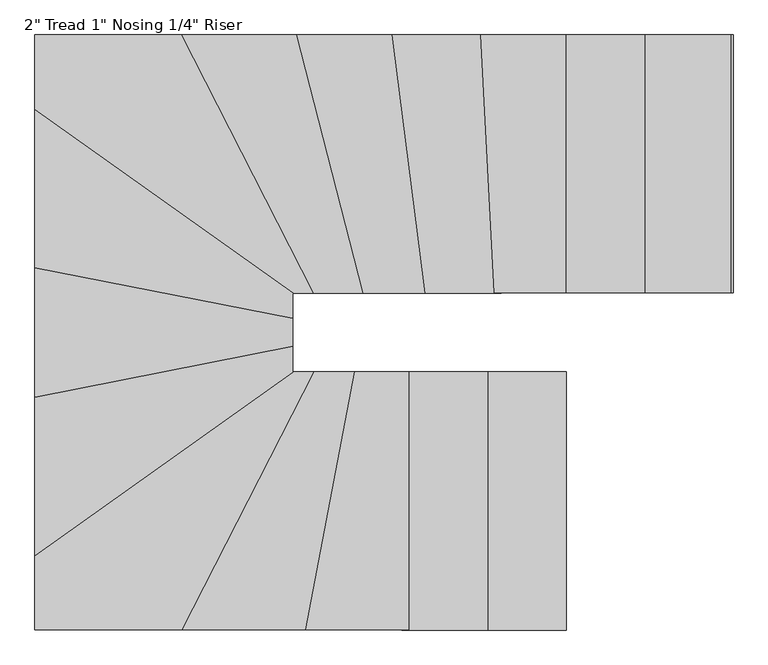
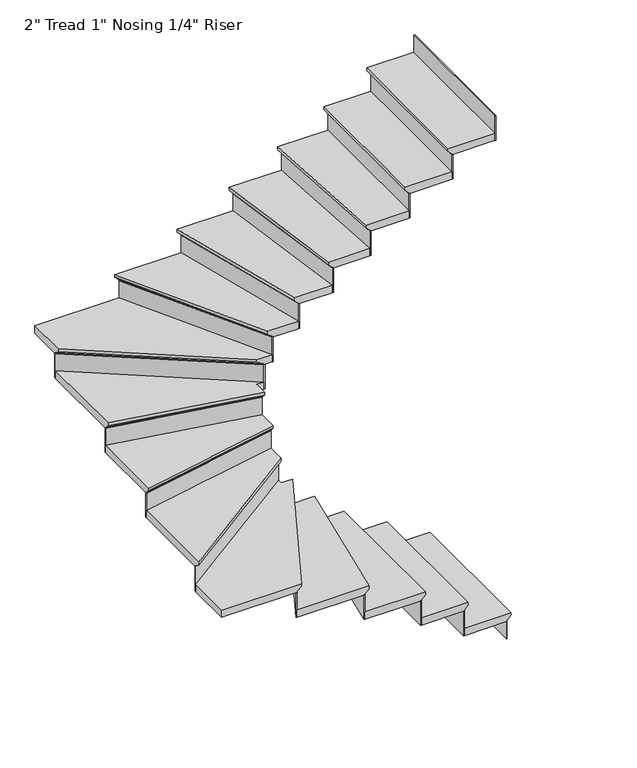
"""IFC4 building model written with IfcOpenShell, lengths in millimetres: stair flight geometry."""

from ifc_helpers import new_model, si_unit, origin, place, context, project, spatial, faceted_brep, source, transform, mapped, element, save


def stair_flight_5a50a9e8(model_context):
    return source(origin(), model_context, "Body", "Brep", [
        faceted_brep([(-8420.1659688, 2083.499435, 488.95), (-8420.1659688, 2083.499435, 508.0), (-8420.1659688, 1169.099435, 508.0), (-8420.1659688, 1169.099435, 488.95), (-8445.5659688, 2083.499435, 463.55), (-8445.5659688, 1169.099435, 463.55), (-8724.9659688, 2083.499435, 508.0), (-8724.9659688, 1169.099435, 508.0), (-8445.5659688, 1169.099435, 457.2), (-8724.9659688, 1169.099435, 457.2), (-8724.9659688, 2083.499435, 457.2), (-8445.5659688, 2083.499435, 457.2)], [[[0, 1, 2, 3]], [[4, 0, 3, 5]], [[2, 1, 6, 7]], [[8, 9, 10, 11]], [[2, 7, 9, 8, 5, 3]], [[8, 11, 4, 5]], [[6, 1, 0, 4, 11, 10]], [[7, 6, 10, 9]]]),
        faceted_brep([(-8445.5659688, 2083.499435, 457.2), (-8445.5659688, 2083.499435, 338.6666667), (-8451.9159688, 2083.499435, 338.6666667), (-8451.9159688, 2083.499435, 457.2), (-8445.5659688, 1169.099435, 457.2), (-8451.9159688, 1169.099435, 457.2), (-8451.9159688, 1169.099435, 338.6666667), (-8445.5659688, 1169.099435, 338.6666667)], [[[0, 1, 2, 3]], [[4, 5, 6, 7]], [[1, 0, 4, 7]], [[2, 1, 7, 6]], [[3, 2, 6, 5]], [[0, 3, 5, 4]]]),
        faceted_brep([(-8724.9659688, 2083.499435, 626.5333333), (-8724.9659688, 2083.499435, 457.2), (-8731.3159688, 2083.499435, 457.2), (-8731.3159688, 2083.499435, 626.5333333), (-8724.9659688, 1169.099435, 626.5333333), (-8731.3159688, 1169.099435, 626.5333333), (-8731.3159688, 1169.099435, 457.2), (-8724.9659688, 1169.099435, 457.2)], [[[0, 1, 2, 3]], [[4, 5, 6, 7]], [[1, 0, 4, 7]], [[2, 1, 7, 6]], [[3, 2, 6, 5]], [[0, 3, 5, 4]]]),
        faceted_brep([(-8699.5659688, 1169.099435, 677.3333333), (-8699.5659688, 2083.499435, 677.3333333), (-9004.3659688, 2083.499435, 677.3333333), (-9004.3659688, 1169.099435, 677.3333333), (-8724.9659688, 1169.099435, 626.5333333), (-9004.3659688, 1169.099435, 626.5333333), (-9004.3659688, 2083.499435, 626.5333333), (-8724.9659688, 2083.499435, 626.5333333), (-8724.9659688, 1169.099435, 632.8833333), (-8699.5659688, 1169.099435, 658.2833333), (-8724.9659688, 2083.499435, 632.8833333), (-8699.5659688, 2083.499435, 658.2833333)], [[[0, 1, 2, 3]], [[4, 5, 6, 7]], [[0, 3, 5, 4, 8, 9]], [[4, 7, 10, 8]], [[2, 1, 11, 10, 7, 6]], [[3, 2, 6, 5]], [[11, 1, 0, 9]], [[10, 11, 9, 8]]]),
        faceted_brep([(-9004.3659688, 2083.499435, 795.8666667), (-9004.3659688, 2083.499435, 626.5333333), (-9010.7159688, 2083.499435, 626.5333333), (-9010.7159688, 2083.499435, 795.8666667), (-9004.3659688, 1169.099435, 795.8666667), (-9010.7159688, 1169.099435, 795.8666667), (-9010.7159688, 1169.099435, 626.5333333), (-9004.3659688, 1169.099435, 626.5333333)], [[[0, 1, 2, 3]], [[4, 5, 6, 7]], [[1, 0, 4, 7]], [[2, 1, 7, 6]], [[3, 2, 6, 5]], [[0, 3, 5, 4]]]),
        faceted_brep([(-8978.9659688, 1169.099435, 846.6666667), (-8978.9659688, 2083.499435, 846.6666667), (-9197.7461084, 2083.499435, 846.6666667), (-9370.6864067, 1169.099435, 846.6666667), (-9004.3659688, 1169.099435, 795.8666667), (-9370.6864067, 1169.099435, 795.8666667), (-9197.7461084, 2083.499435, 795.8666667), (-9004.3659688, 2083.499435, 795.8666667), (-9004.3659688, 1169.099435, 802.2166667), (-8978.9659688, 1169.099435, 827.6166667), (-9004.3659688, 2083.499435, 802.2166667), (-8978.9659688, 2083.499435, 827.6166667)], [[[0, 1, 2, 3]], [[4, 5, 6, 7]], [[0, 3, 5, 4, 8, 9]], [[4, 7, 10, 8]], [[2, 1, 11, 10, 7, 6]], [[3, 2, 6, 5]], [[11, 1, 0, 9]], [[10, 11, 9, 8]]]),
        faceted_brep([(-9197.7461084, 2083.499435, 965.2), (-9197.7461084, 2083.499435, 795.8666667), (-9204.2086806, 2083.499435, 795.8666667), (-9204.2086806, 2083.499435, 965.2), (-9370.6864067, 1169.099435, 965.2), (-9377.1489789, 1169.099435, 965.2), (-9377.1489789, 1169.099435, 795.8666667), (-9370.6864067, 1169.099435, 795.8666667)], [[[0, 1, 2, 3]], [[4, 5, 6, 7]], [[1, 0, 4, 7]], [[2, 1, 7, 6]], [[3, 2, 6, 5]], [[0, 3, 5, 4]]]),
        faceted_brep([(-9344.836118, 1169.099435, 1016.0), (-9171.8958196, 2083.499435, 1016.0), (-9343.3736886, 2083.499435, 1016.0), (-9812.19831, 1169.099435, 1016.0), (-9370.6864067, 1169.099435, 965.2), (-9812.19831, 1169.099435, 965.2), (-9343.3736886, 2083.499435, 965.2), (-9197.7461084, 2083.499435, 965.2), (-9370.6864067, 1169.099435, 971.55), (-9344.836118, 1169.099435, 996.95), (-9197.7461084, 2083.499435, 971.55), (-9171.8958196, 2083.499435, 996.95)], [[[0, 1, 2, 3]], [[4, 5, 6, 7]], [[0, 3, 5, 4, 8, 9]], [[4, 7, 10, 8]], [[2, 1, 11, 10, 7, 6]], [[3, 2, 6, 5]], [[11, 1, 0, 9]], [[10, 11, 9, 8]]]),
        faceted_brep([(-9343.3736886, 2083.499435, 1134.5333333), (-9343.3736886, 2083.499435, 965.2), (-9350.5096718, 2083.499435, 965.2), (-9350.5096718, 2083.499435, 1134.5333333), (-9812.19831, 1169.099435, 1134.5333333), (-9819.3342931, 1169.099435, 1134.5333333), (-9819.3342931, 1169.099435, 965.2), (-9812.19831, 1169.099435, 965.2)], [[[0, 1, 2, 3]], [[4, 5, 6, 7]], [[1, 0, 4, 7]], [[2, 1, 7, 6]], [[3, 2, 6, 5]], [[0, 3, 5, 4]]]),
        faceted_brep([(-10303.4976606, 1462.7805687, 1185.3333333), (-10303.4976606, 1169.099435, 1185.3333333), (-9783.6543774, 1169.099435, 1185.3333333), (-9314.8297561, 2083.499435, 1185.3333333), (-9389.0976606, 2083.499435, 1185.3333333), (-9389.0976606, 2113.0545178, 1185.3333333), (-10303.4976606, 1169.099435, 1134.5333333), (-10303.4976606, 1462.7805687, 1134.5333333), (-9389.0976606, 2113.0545178, 1134.5333333), (-9389.0976606, 2083.499435, 1134.5333333), (-9343.3736886, 2083.499435, 1134.5333333), (-9812.19831, 1169.099435, 1134.5333333), (-9343.3736886, 2083.499435, 1140.8833333), (-9812.19831, 1169.099435, 1140.8833333), (-9314.8297561, 2083.499435, 1166.2833333), (-9783.6543774, 1169.099435, 1166.2833333)], [[[0, 1, 2, 3, 4, 5]], [[6, 7, 8, 9, 10, 11]], [[1, 0, 7, 6]], [[11, 10, 12, 13]], [[4, 3, 14, 12, 10, 9]], [[0, 5, 8, 7]], [[14, 3, 2, 15]], [[12, 14, 15, 13]], [[2, 1, 6, 11, 13, 15]], [[5, 4, 9, 8]]]),
        faceted_brep([(-9389.0976606, 2113.0545178, 1303.8666667), (-9389.0976606, 2113.0545178, 1134.5333333), (-9389.0976606, 2120.8464926, 1134.5333333), (-9389.0976606, 2120.8464926, 1303.8666667), (-10303.4976606, 1462.7805687, 1303.8666667), (-10303.4976606, 1470.5725435, 1303.8666667), (-10303.4976606, 1470.5725435, 1134.5333333), (-10303.4976606, 1462.7805687, 1134.5333333)], [[[0, 1, 2, 3]], [[4, 5, 6, 7]], [[1, 0, 4, 7]], [[2, 1, 7, 6]], [[3, 2, 6, 5]], [[0, 3, 5, 4]]]),
        faceted_brep([(-10303.4976606, 1431.6126695, 1354.6666667), (-9389.0976606, 2081.8866187, 1354.6666667), (-9389.0976606, 2199.5086049, 1354.6666667), (-10303.4976606, 2019.2677486, 1354.6666667), (-10303.4976606, 1462.7805687, 1303.8666667), (-10303.4976606, 2019.2677486, 1303.8666667), (-9389.0976606, 2199.5086049, 1303.8666667), (-9389.0976606, 2113.0545178, 1303.8666667), (-10303.4976606, 1462.7805687, 1310.2166667), (-10303.4976606, 1431.6126695, 1335.6166667), (-9389.0976606, 2113.0545178, 1310.2166667), (-9389.0976606, 2081.8866187, 1335.6166667)], [[[0, 1, 2, 3]], [[4, 5, 6, 7]], [[0, 3, 5, 4, 8, 9]], [[4, 7, 10, 8]], [[3, 2, 6, 5]], [[11, 1, 0, 9]], [[10, 11, 9, 8]], [[2, 1, 11, 10, 7, 6]]]),
        faceted_brep([(-9389.0976606, 2199.5086049, 1473.2), (-9389.0976606, 2199.5086049, 1303.8666667), (-9389.0976606, 2205.9807903, 1303.8666667), (-9389.0976606, 2205.9807903, 1473.2), (-10303.4976606, 2019.2677486, 1473.2), (-10303.4976606, 2025.739934, 1473.2), (-10303.4976606, 2025.739934, 1303.8666667), (-10303.4976606, 2019.2677486, 1303.8666667)], [[[0, 1, 2, 3]], [[4, 5, 6, 7]], [[1, 0, 4, 7]], [[2, 1, 7, 6]], [[3, 2, 6, 5]], [[0, 3, 5, 4]]]),
        faceted_brep([(-10303.4976606, 1993.3790068, 1524.0), (-9389.0976606, 2173.6198632, 1524.0), (-9389.0976606, 2298.6677486, 1524.0), (-10303.4976606, 2478.9086049, 1524.0), (-10303.4976606, 2019.2677486, 1473.2), (-10303.4976606, 2478.9086049, 1473.2), (-9389.0976606, 2298.6677486, 1473.2), (-9389.0976606, 2199.5086049, 1473.2), (-10303.4976606, 2019.2677486, 1479.55), (-10303.4976606, 1993.3790068, 1504.95), (-9389.0976606, 2199.5086049, 1479.55), (-9389.0976606, 2173.6198632, 1504.95)], [[[0, 1, 2, 3]], [[4, 5, 6, 7]], [[0, 3, 5, 4, 8, 9]], [[4, 7, 10, 8]], [[2, 1, 11, 10, 7, 6]], [[3, 2, 6, 5]], [[11, 1, 0, 9]], [[10, 11, 9, 8]]]),
        faceted_brep([(-9389.0976606, 2298.6677486, 1642.5333333), (-9389.0976606, 2298.6677486, 1473.2), (-9389.0976606, 2305.139934, 1473.2), (-9389.0976606, 2305.139934, 1642.5333333), (-10303.4976606, 2478.9086049, 1642.5333333), (-10303.4976606, 2485.3807903, 1642.5333333), (-10303.4976606, 2485.3807903, 1473.2), (-10303.4976606, 2478.9086049, 1473.2)], [[[0, 1, 2, 3]], [[4, 5, 6, 7]], [[1, 0, 4, 7]], [[2, 1, 7, 6]], [[3, 2, 6, 5]], [[0, 3, 5, 4]]]),
        faceted_brep([(-10303.4976606, 2453.0198632, 1693.3333333), (-9389.0976606, 2272.7790068, 1693.3333333), (-9389.0976606, 2362.899435, 1693.3333333), (-9343.0021861, 2362.899435, 1693.3333333), (-10303.4976606, 3045.9540996, 1693.3333333), (-10303.4976606, 2478.9086049, 1642.5333333), (-10303.4976606, 3045.9540996, 1642.5333333), (-9343.0021861, 2362.899435, 1642.5333333), (-9389.0976606, 2362.899435, 1642.5333333), (-9389.0976606, 2298.6677486, 1642.5333333), (-10303.4976606, 2478.9086049, 1648.8833333), (-10303.4976606, 2453.0198632, 1674.2833333), (-9389.0976606, 2298.6677486, 1648.8833333), (-9389.0976606, 2272.7790068, 1674.2833333)], [[[0, 1, 2, 3, 4]], [[5, 6, 7, 8, 9]], [[0, 4, 6, 5, 10, 11]], [[5, 9, 12, 10]], [[3, 2, 8, 7]], [[4, 3, 7, 6]], [[13, 1, 0, 11]], [[12, 13, 11, 10]], [[2, 1, 13, 12, 9, 8]]]),
        faceted_brep([(-9343.0021861, 2362.899435, 1811.8666667), (-9343.0021861, 2362.899435, 1642.5333333), (-9332.0452936, 2362.899435, 1642.5333333), (-9332.0452936, 2362.899435, 1811.8666667), (-10303.4976606, 3045.9540996, 1811.8666667), (-10303.4976606, 3053.7460744, 1811.8666667), (-10303.4976606, 3053.7460744, 1642.5333333), (-10303.4976606, 3045.9540996, 1642.5333333)], [[[0, 1, 2, 3]], [[4, 5, 6, 7]], [[1, 0, 4, 7]], [[2, 1, 7, 6]], [[3, 2, 6, 5]], [[0, 3, 5, 4]]]),
        faceted_brep([(-9755.1104449, 3277.299435, 1862.6666667), (-10303.4976606, 3277.299435, 1862.6666667), (-10303.4976606, 3014.7862005, 1862.6666667), (-9386.8297561, 2362.899435, 1862.6666667), (-9286.2858236, 2362.899435, 1862.6666667), (-10303.4976606, 3277.299435, 1811.8666667), (-9755.1104449, 3277.299435, 1811.8666667), (-9286.2858236, 2362.899435, 1811.8666667), (-9343.0021861, 2362.899435, 1811.8666667), (-10303.4976606, 3045.9540996, 1811.8666667), (-9343.0021861, 2362.899435, 1818.2166667), (-10303.4976606, 3045.9540996, 1818.2166667), (-9386.8297561, 2362.899435, 1843.6166667), (-10303.4976606, 3014.7862005, 1843.6166667)], [[[0, 1, 2, 3, 4]], [[5, 6, 7, 8, 9]], [[1, 0, 6, 5]], [[9, 8, 10, 11]], [[4, 3, 12, 10, 8, 7]], [[0, 4, 7, 6]], [[12, 3, 2, 13]], [[10, 12, 13, 11]], [[2, 1, 5, 9, 11, 13]]]),
        faceted_brep([(-9286.2858236, 2362.899435, 1981.2), (-9286.2858236, 2362.899435, 1811.8666667), (-9279.1498404, 2362.899435, 1811.8666667), (-9279.1498404, 2362.899435, 1981.2), (-9755.1104449, 3277.299435, 1981.2), (-9747.9744618, 3277.299435, 1981.2), (-9747.9744618, 3277.299435, 1811.8666667), (-9755.1104449, 3277.299435, 1811.8666667)], [[[0, 1, 2, 3]], [[4, 5, 6, 7]], [[1, 0, 4, 7]], [[2, 1, 7, 6]], [[3, 2, 6, 5]], [[0, 3, 5, 4]]]),
        faceted_brep([(-9783.6543774, 3277.299435, 2032.0), (-9314.8297561, 2362.899435, 2032.0), (-9114.5744376, 2362.899435, 2032.0), (-9349.704885, 3277.299435, 2032.0), (-9755.1104449, 3277.299435, 1981.2), (-9349.704885, 3277.299435, 1981.2), (-9114.5744376, 2362.899435, 1981.2), (-9286.2858236, 2362.899435, 1981.2), (-9755.1104449, 3277.299435, 1987.55), (-9783.6543774, 3277.299435, 2012.95), (-9286.2858236, 2362.899435, 1987.55), (-9314.8297561, 2362.899435, 2012.95)], [[[0, 1, 2, 3]], [[4, 5, 6, 7]], [[0, 3, 5, 4, 8, 9]], [[4, 7, 10, 8]], [[2, 1, 11, 10, 7, 6]], [[3, 2, 6, 5]], [[11, 1, 0, 9]], [[10, 11, 9, 8]]]),
        faceted_brep([(-9114.5744376, 2362.899435, 2150.5333333), (-9114.5744376, 2362.899435, 1981.2), (-9108.0178608, 2362.899435, 1981.2), (-9108.0178608, 2362.899435, 2150.5333333), (-9349.704885, 3277.299435, 2150.5333333), (-9343.1483082, 3277.299435, 2150.5333333), (-9343.1483082, 3277.299435, 1981.2), (-9349.704885, 3277.299435, 1981.2)], [[[0, 1, 2, 3]], [[4, 5, 6, 7]], [[1, 0, 4, 7]], [[2, 1, 7, 6]], [[3, 2, 6, 5]], [[0, 3, 5, 4]]]),
        faceted_brep([(-9375.9311925, 3277.299435, 2201.3333333), (-9140.8007451, 2362.899435, 2201.3333333), (-8894.1760558, 2362.899435, 2201.3333333), (-9012.5321075, 3277.299435, 2201.3333333), (-9349.704885, 3277.299435, 2150.5333333), (-9012.5321075, 3277.299435, 2150.5333333), (-8894.1760558, 2362.899435, 2150.5333333), (-9114.5744376, 2362.899435, 2150.5333333), (-9349.704885, 3277.299435, 2156.8833333), (-9375.9311925, 3277.299435, 2182.2833333), (-9114.5744376, 2362.899435, 2156.8833333), (-9140.8007451, 2362.899435, 2182.2833333)], [[[0, 1, 2, 3]], [[4, 5, 6, 7]], [[0, 3, 5, 4, 8, 9]], [[4, 7, 10, 8]], [[2, 1, 11, 10, 7, 6]], [[3, 2, 6, 5]], [[11, 1, 0, 9]], [[10, 11, 9, 8]]]),
        faceted_brep([(-8894.1760558, 2362.899435, 2319.8666667), (-8894.1760558, 2362.899435, 2150.5333333), (-8887.7730841, 2362.899435, 2150.5333333), (-8887.7730841, 2362.899435, 2319.8666667), (-9012.5321075, 3277.299435, 2319.8666667), (-9006.1291357, 3277.299435, 2319.8666667), (-9006.1291357, 3277.299435, 2150.5333333), (-9012.5321075, 3277.299435, 2150.5333333)], [[[0, 1, 2, 3]], [[4, 5, 6, 7]], [[1, 0, 4, 7]], [[2, 1, 7, 6]], [[3, 2, 6, 5]], [[0, 3, 5, 4]]]),
        faceted_brep([(-9038.1439946, 3277.299435, 2370.6666667), (-8919.787943, 2362.899435, 2370.6666667), (-8650.3645369, 2362.899435, 2370.6666667), (-8697.8988073, 3277.299435, 2370.6666667), (-9012.5321075, 3277.299435, 2319.8666667), (-8697.8988073, 3277.299435, 2319.8666667), (-8650.3645369, 2362.899435, 2319.8666667), (-8894.1760558, 2362.899435, 2319.8666667), (-9012.5321075, 3277.299435, 2326.2166667), (-9038.1439946, 3277.299435, 2351.6166667), (-8894.1760558, 2362.899435, 2326.2166667), (-8919.787943, 2362.899435, 2351.6166667)], [[[0, 1, 2, 3]], [[4, 5, 6, 7]], [[0, 3, 5, 4, 8, 9]], [[4, 7, 10, 8]], [[2, 1, 11, 10, 7, 6]], [[3, 2, 6, 5]], [[11, 1, 0, 9]], [[10, 11, 9, 8]]]),
        faceted_brep([(-8650.3645369, 2362.899435, 2489.2), (-8650.3645369, 2362.899435, 2319.8666667), (-8644.0059628, 2362.899435, 2319.8666667), (-8644.0059628, 2362.899435, 2489.2), (-8697.8988073, 3277.299435, 2489.2), (-8691.5402332, 3277.299435, 2489.2), (-8691.5402332, 3277.299435, 2319.8666667), (-8697.8988073, 3277.299435, 2319.8666667)], [[[0, 1, 2, 3]], [[4, 5, 6, 7]], [[1, 0, 4, 7]], [[2, 1, 7, 6]], [[3, 2, 6, 5]], [[0, 3, 5, 4]]]),
        faceted_brep([(-8723.333104, 3277.299435, 2540.0), (-8675.7988336, 2362.899435, 2540.0), (-8394.7659688, 2362.899435, 2540.0), (-8394.7659688, 3277.299435, 2540.0), (-8697.8988073, 3277.299435, 2489.2), (-8394.7659688, 3277.299435, 2489.2), (-8394.7659688, 2362.899435, 2489.2), (-8650.3645369, 2362.899435, 2489.2), (-8697.8988073, 3277.299435, 2495.55), (-8723.333104, 3277.299435, 2520.95), (-8650.3645369, 2362.899435, 2495.55), (-8675.7988336, 2362.899435, 2520.95)], [[[0, 1, 2, 3]], [[4, 5, 6, 7]], [[0, 3, 5, 4, 8, 9]], [[4, 7, 10, 8]], [[2, 1, 11, 10, 7, 6]], [[3, 2, 6, 5]], [[11, 1, 0, 9]], [[10, 11, 9, 8]]]),
        faceted_brep([(-8394.7659688, 2362.899435, 2658.5333333), (-8394.7659688, 2362.899435, 2489.2), (-8388.4159688, 2362.899435, 2489.2), (-8388.4159688, 2362.899435, 2658.5333333), (-8394.7659688, 3277.299435, 2658.5333333), (-8388.4159688, 3277.299435, 2658.5333333), (-8388.4159688, 3277.299435, 2489.2), (-8394.7659688, 3277.299435, 2489.2)], [[[0, 1, 2, 3]], [[4, 5, 6, 7]], [[1, 0, 4, 7]], [[2, 1, 7, 6]], [[3, 2, 6, 5]], [[0, 3, 5, 4]]]),
        faceted_brep([(-8420.1659688, 3277.299435, 2709.3333333), (-8420.1659688, 2362.899435, 2709.3333333), (-8115.3659688, 2362.899435, 2709.3333333), (-8115.3659688, 3277.299435, 2709.3333333), (-8394.7659688, 3277.299435, 2658.5333333), (-8115.3659688, 3277.299435, 2658.5333333), (-8115.3659688, 2362.899435, 2658.5333333), (-8394.7659688, 2362.899435, 2658.5333333), (-8394.7659688, 3277.299435, 2664.8833333), (-8420.1659688, 3277.299435, 2690.2833333), (-8394.7659688, 2362.899435, 2664.8833333), (-8420.1659688, 2362.899435, 2690.2833333)], [[[0, 1, 2, 3]], [[4, 5, 6, 7]], [[0, 3, 5, 4, 8, 9]], [[4, 7, 10, 8]], [[2, 1, 11, 10, 7, 6]], [[3, 2, 6, 5]], [[11, 1, 0, 9]], [[10, 11, 9, 8]]]),
        faceted_brep([(-8115.3659688, 2362.899435, 2827.8666667), (-8115.3659688, 2362.899435, 2658.5333333), (-8109.0159688, 2362.899435, 2658.5333333), (-8109.0159688, 2362.899435, 2827.8666667), (-8115.3659688, 3277.299435, 2827.8666667), (-8109.0159688, 3277.299435, 2827.8666667), (-8109.0159688, 3277.299435, 2658.5333333), (-8115.3659688, 3277.299435, 2658.5333333)], [[[0, 1, 2, 3]], [[4, 5, 6, 7]], [[1, 0, 4, 7]], [[2, 1, 7, 6]], [[3, 2, 6, 5]], [[0, 3, 5, 4]]]),
        faceted_brep([(-7835.9659688, 2362.899435, 2997.2), (-7835.9659688, 2362.899435, 2827.8666667), (-7829.6159688, 2362.899435, 2827.8666667), (-7829.6159688, 2362.899435, 2997.2), (-7835.9659688, 3277.299435, 2997.2), (-7829.6159688, 3277.299435, 2997.2), (-7829.6159688, 3277.299435, 2827.8666667), (-7835.9659688, 3277.299435, 2827.8666667)], [[[0, 1, 2, 3]], [[4, 5, 6, 7]], [[1, 0, 4, 7]], [[2, 1, 7, 6]], [[3, 2, 6, 5]], [[0, 3, 5, 4]]]),
        faceted_brep([(-8140.7659688, 3277.299435, 2878.6666667), (-8140.7659688, 2362.899435, 2878.6666667), (-7835.9659688, 2362.899435, 2878.6666667), (-7835.9659688, 3277.299435, 2878.6666667), (-8115.3659688, 3277.299435, 2827.8666667), (-7835.9659688, 3277.299435, 2827.8666667), (-7835.9659688, 2362.899435, 2827.8666667), (-8115.3659688, 2362.899435, 2827.8666667), (-8115.3659688, 3277.299435, 2834.2166667), (-8140.7659688, 3277.299435, 2859.6166667), (-8115.3659688, 2362.899435, 2834.2166667), (-8140.7659688, 2362.899435, 2859.6166667)], [[[0, 1, 2, 3]], [[4, 5, 6, 7]], [[0, 3, 5, 4, 8, 9]], [[4, 7, 10, 8]], [[2, 1, 11, 10, 7, 6]], [[3, 2, 6, 5]], [[11, 1, 0, 9]], [[10, 11, 9, 8]]]),
    ])


if __name__ == "__main__":
    model = new_model("IFC4")
    model_context = context("Model", 3, world=origin())
    ifc_project = project(units=[si_unit("LENGTHUNIT", "METRE", prefix="MILLI")], contexts=[model_context])
    site = spatial("IfcSite", under=ifc_project)
    building = spatial("IfcBuilding", under=site)
    placement = place(None, origin())
    stair_flight_shape = stair_flight_5a50a9e8(model_context)
    element("IfcStairFlight", 1, ObjectType="2\" Tread 1\" Nosing 1/4\" Riser", at=placement, inside=building, context=model_context, shape_type="MappedRepresentation", body=[
        mapped(stair_flight_shape, transform((0.0, 0.0, 0.0), x_axis=(1.0, 0.0, 0.0), y_axis=(0.0, 1.0, 0.0), z_axis=(0.0, 0.0, 1.0))),
    ])
    save(model, "model.ifc")
